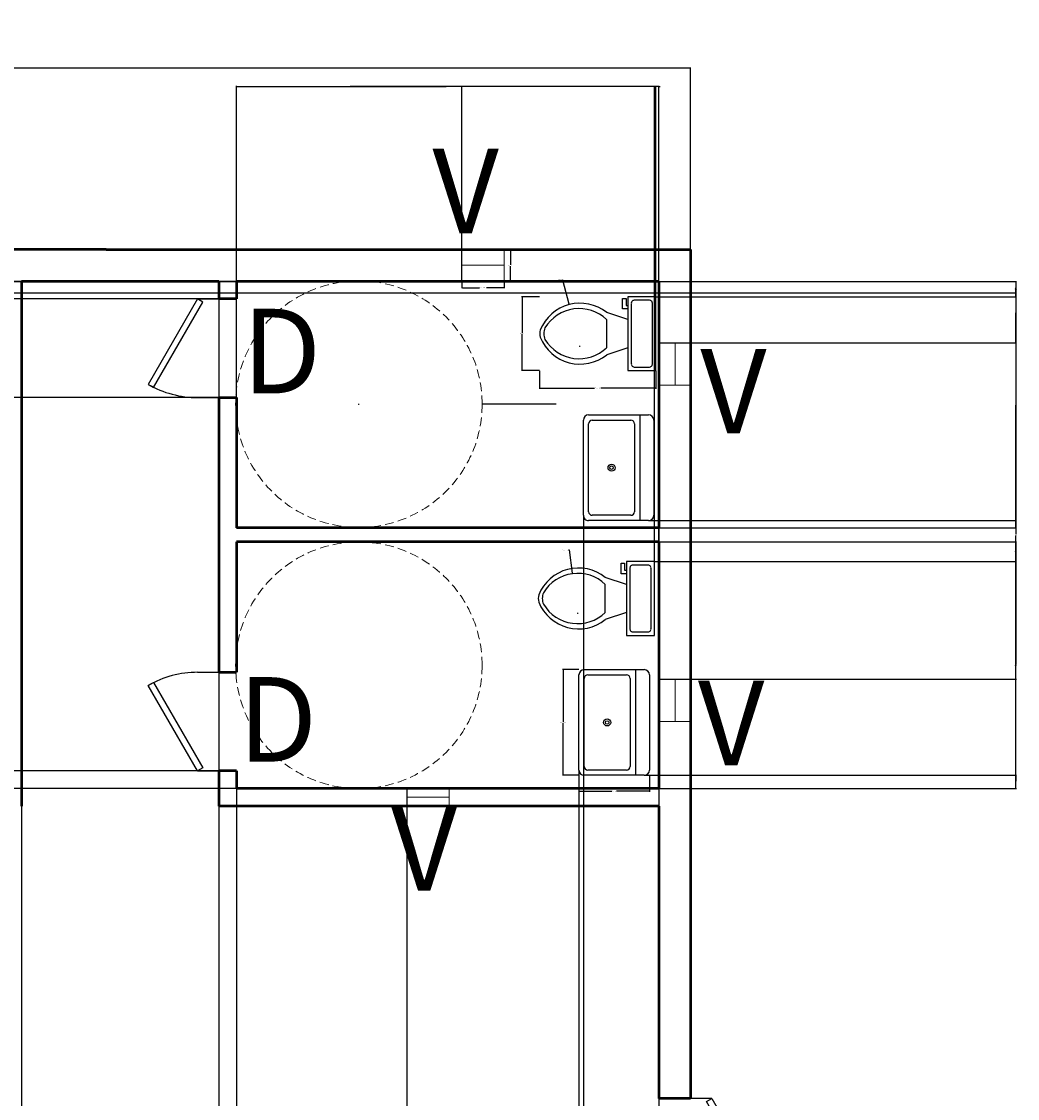
# Model space of a CAD drawing. Units: inches. Extents: x -84 to 931, y 65 to 668.
# Tile 5 of 5: x 649 to 931, y 363 to 668. Entities that reach past the tile are written whole.
import ezdxf

# ---------------------------------------------------------------- set-up
doc = ezdxf.new("R2010")
doc.units = ezdxf.units.IN
doc.header["$MEASUREMENT"] = 0
doc.linetypes.add('HIDDEN', pattern=[0.375, 0.25, -0.125])
for name, color, linetype, lineweight in [('A-ANNO-DIMS', 2, 'Continuous', 18), ('A-ANNO-TEXT', 7, 'Continuous', 18), ('A-DOOR', 4, 'Continuous', 25), ('A-FLOR-CLRN', 8, 'HIDDEN', 13), ('A-FLOR-FIXT', 9, 'Continuous', 25), ('A-GLAZ-VENT', 3, 'Continuous', 18), ('A-WALL', 7, 'Continuous', 50)]:
    doc.layers.add(name, color=color, linetype=linetype, lineweight=lineweight)
doc.styles.get("Standard").update_dxf_attribs({"font": 'arial.ttf'})
doc.dimstyles.get("Standard").update_dxf_attribs({"dimtxt": 0.18, "dimasz": 0.18, "dimexe": 0.18, "dimexo": 0.0625, "dimgap": 0.09, "dimtad": 0, "dimtih": 1, "dimtoh": 1, "dimdec": 0, "dimzin": 0, "dimdsep": 46, "dimlunit": 3, "dimtxsty": 'Standard', "dimcen": 0.09, "dimadec": 0, "dimazin": 0, "dimtfac": 1, "dimtdec": 0, "dimtofl": 0, "dimtmove": 0, "dimatfit": 3, "dimfxl": 1, "dimtolj": 1, "dimtzin": 0, "dimarcsym": 0})

# ---------------------------------------------------------------- blocks, each defined once
blk = doc.blocks.new('*U5')
for p, q in [((0, 0), (0, -6)), ((-28, 0), (-28, -6))]:
    blk.add_line(p, q)
blk.add_lwpolyline([(0, 0), (-24.25, 14), (-25.12, 12.48), (-0.87, -1.52)], close=True)
blk.add_arc((0, 0), 28, 150, 180)
blk = doc.blocks.new('*U6')
for p, q in [((0, 0), (0, -6)), ((28, 0), (28, -6))]:
    blk.add_line(p, q)
blk.add_lwpolyline([(0, 0), (24.25, 14), (25.12, 12.48), (0.87, -1.52)], close=True)
blk.add_arc((0, 0), 28, 0, 30)
blk = doc.blocks.new('*U13')
for p, q in [((-40, 0), (-40, 6)), ((0, 0), (0, 6))]:
    blk.add_line(p, q)
blk.add_lwpolyline([(0, 0), (-34.64, -20), (-35.52, -18.48), (-0.87, 1.52)], close=True)
blk.add_arc((0, 0), 40, 180, 210)
blk = doc.blocks.new('Sink-single - 30 in top')
blk.add_line((-15, -3.999996), (15, -3.999996))
for points in [[(-13.5, 0), (13.5, 0)], [(-15, -18.499996), (-15, -1.5)], [(15, -1.5), (15, -18.499996)], [(-12.5, -5.499996), (12.5, -5.499996)], [(-13.5, -17.499996), (-13.5, -6.499996)], [(13.5, -6.499996), (13.5, -17.499996)], [(13.5, -19.999996), (-13.5, -19.999996)], [(12.5, -18.499996), (-12.5, -18.499996)]]:
    blk.add_lwpolyline(points)
for radius in [1, 0.5]:
    blk.add_circle((0, -11.999996), radius)
for centre, radius, start, end in [((-13.5, -1.5), 1.5, 90, 180), ((13.5, -1.5), 1.5, 0, 90), ((-12.5, -6.499996), 1, 90, 180), ((12.5, -6.499996), 1, 0, 90), ((-12.5, -17.499996), 1, 180, 270), ((12.5, -17.499996), 1, 270, 0), ((-13.5, -18.499996), 1.5, 180, 270), ((13.5, -18.499996), 1.5, 270, 0)]:
    blk.add_arc(centre, radius, start, end)
blk = doc.blocks.new('Toilet - top')
for p, q in [((9.5, -6), (9.5, -2)), ((-10, -8.5), (-8, -8.5)), ((-10, -9.5), (-10, -8.5)), ((-8, -8.5), (-8, -8)), ((-7, -8), (-7, -9.5)), ((-4, -8), (-6, -14)), ((4, -8), (6, -14)), ((-7, -9.5), (-10, -9.5)), ((4, -14), (-4, -14))]:
    blk.add_line(p, q)
blk.add_lwpolyline([(10.5, -8), (10.5, 0), (-10.5, 0), (-10.5, -8)], close=True)
for points in [[(-9.5, -2), (-9.5, -6)], [(8.5, -1), (-8.5, -1)], [(-8.5, -7), (8.5, -7)]]:
    blk.add_lwpolyline(points)
for centre, radius, start, end in [((-8.62, -1.88), 0.884, 81.8699, 188.1301), ((8.62, -1.88), 0.884, 351.8699, 98.1301), ((-8.62, -6.12), 0.884, 171.8699, 278.1301), ((8.62, -6.12), 0.884, 261.8699, 8.1301), ((3.52, -21.58), 12.17, 141.4691, 247.9714), ((4.2, -21.82), 11.33, 136.3677, 238.9468), ((-3.52, -21.58), 12.17, 292.0284, 38.5307), ((-4.2, -21.82), 11.33, 301.053, 43.6321), ((0, -27.88), 4, 245.7318, 294.2682), ((0, -29), 4, 254.8605, 285.1395)]:
    blk.add_arc(centre, radius, start, end)
blk = doc.blocks.new('*D17')
at = {"layer": 'A-ANNO-DIMS', "color": 0, "lineweight": -2, "transparency": 16777216}
for p, q in [((0.53, 603.58), (0.53, 655.22)), ((0.71, 655.04), (368.83, 655.04)), ((838.35, 655.04), (470.23, 655.04)), ((838.53, 603.58), (838.53, 655.22))]:
    blk.add_line(p, q, dxfattribs=at)
at = {"layer": 'A-ANNO-DIMS', "color": 0, "transparency": 16777216}
for points in [[(0.71, 655.07), (0.71, 655.01), (0.53, 655.04)], [(838.35, 655.07), (838.35, 655.01), (838.53, 655.04)]]:
    blk.add_solid(points, dxfattribs=at)
at = {"layer": 'Defpoints', "color": 0, "transparency": 16777216}
for p in [(838.53, 655.04), (0.53, 603.52), (838.53, 603.52)]:
    blk.add_point(p, dxfattribs=at)
at = {"layer": 'A-ANNO-DIMS', "color": 0, "transparency": 16777216, "insert": (419.53, 655.04), "char_height": 0.18, "attachment_point": 5}
blk.add_mtext('\\A1;{\\H133.33333x;69\'-10"}', dxfattribs=at)
blk = doc.blocks.new('VENT-12IN-EXT')
blk.add_line((0, 4.61), (12, 4.61))
blk.add_lwpolyline([(0, 9), (12, 9), (12, 0), (0, 0)], close=True)
blk = doc.blocks.new('*D23')
at = {"layer": 'A-ANNO-DIMS', "color": 0, "lineweight": -2, "transparency": 16777216}
for p, q in [((795.65, 569.11), (795.65, 564.04)), ((828.69, 569.11), (828.69, 564.04)), ((795.83, 564.22), (811.28, 564.22)), ((828.51, 564.22), (813.06, 564.22))]:
    blk.add_line(p, q, dxfattribs=at)
at = {"layer": 'A-ANNO-DIMS', "color": 0, "transparency": 16777216}
for points in [[(795.83, 564.25), (795.83, 564.19), (795.65, 564.22)], [(828.51, 564.25), (828.51, 564.19), (828.69, 564.22)]]:
    blk.add_solid(points, dxfattribs=at)
at = {"layer": 'Defpoints', "color": 0, "transparency": 16777216}
for p in [(795.65, 569.17), (828.69, 569.17), (828.69, 564.22)]:
    blk.add_point(p, dxfattribs=at)
at = {"layer": 'A-ANNO-DIMS', "color": 0, "transparency": 16777216, "insert": (812.17, 564.22), "char_height": 0.18, "attachment_point": 5}
blk.add_mtext('\\A1;WC 2\'-9" TYP.', dxfattribs=at)
blk = doc.blocks.new('*D24')
at = {"layer": 'A-ANNO-DIMS', "color": 0, "lineweight": -2, "transparency": 16777216}
for p, q in [((795.58, 590.17), (790.51, 590.17)), ((790.69, 589.99), (790.69, 579.85)), ((790.69, 569.35), (790.69, 579.49)), ((795.58, 569.17), (790.51, 569.17))]:
    blk.add_line(p, q, dxfattribs=at)
at = {"layer": 'A-ANNO-DIMS', "color": 0, "transparency": 16777216}
for points in [[(790.66, 589.99), (790.72, 589.99), (790.69, 590.17)], [(790.66, 569.35), (790.72, 569.35), (790.69, 569.17)]]:
    blk.add_solid(points, dxfattribs=at)
at = {"layer": 'Defpoints', "color": 0, "transparency": 16777216}
for p in [(795.65, 590.17), (790.69, 569.17), (795.65, 569.17)]:
    blk.add_point(p, dxfattribs=at)
at = {"layer": 'A-ANNO-DIMS', "color": 0, "transparency": 16777216, "insert": (790.69, 579.67), "char_height": 0.18, "attachment_point": 5}
blk.add_mtext('\\A1;1\'-9" TYP.', dxfattribs=at)
blk = doc.blocks.new('*D25')
at = {"layer": 'A-ANNO-DIMS', "color": 0, "lineweight": -2, "transparency": 16777216}
for p, q in [((773.54, 594.45), (773.54, 592.54)), ((785.54, 594.45), (785.54, 592.54)), ((773.72, 592.72), (778.53, 592.72)), ((785.36, 592.72), (780.55, 592.72))]:
    blk.add_line(p, q, dxfattribs=at)
at = {"layer": 'A-ANNO-DIMS', "color": 0, "transparency": 16777216}
for points in [[(773.72, 592.75), (773.72, 592.69), (773.54, 592.72)], [(785.36, 592.75), (785.36, 592.69), (785.54, 592.72)]]:
    blk.add_solid(points, dxfattribs=at)
at = {"layer": 'Defpoints', "color": 0, "transparency": 16777216}
for p in [(773.54, 594.52), (785.54, 594.52), (785.54, 592.72)]:
    blk.add_point(p, dxfattribs=at)
at = {"layer": 'A-ANNO-DIMS', "color": 0, "transparency": 16777216, "insert": (779.54, 592.72), "char_height": 0.18, "attachment_point": 5}
blk.add_mtext('\\A1;VENT 1\'-0" TYP.', dxfattribs=at)
blk = doc.blocks.new('*D26')
at = {"layer": 'A-ANNO-DIMS', "color": 0, "lineweight": -2, "transparency": 16777216}
for p, q in [((785.6, 603.52), (787.52, 603.52)), ((787.34, 603.34), (787.34, 599.2)), ((787.34, 594.7), (787.34, 598.83)), ((785.6, 594.52), (787.52, 594.52))]:
    blk.add_line(p, q, dxfattribs=at)
at = {"layer": 'A-ANNO-DIMS', "color": 0, "transparency": 16777216}
for points in [[(787.31, 603.34), (787.37, 603.34), (787.34, 603.52)], [(787.31, 594.7), (787.37, 594.7), (787.34, 594.52)]]:
    blk.add_solid(points, dxfattribs=at)
at = {"layer": 'Defpoints', "color": 0, "transparency": 16777216}
for p in [(785.54, 603.52), (787.34, 603.52), (785.54, 594.52)]:
    blk.add_point(p, dxfattribs=at)
at = {"layer": 'A-ANNO-DIMS', "color": 0, "transparency": 16777216, "insert": (787.34, 599.02), "char_height": 0.18, "attachment_point": 5}
blk.add_mtext('\\A1;0\'-9" TYP.', dxfattribs=at)
blk = doc.blocks.new('*D27')
at = {"layer": 'A-ANNO-DIMS', "color": 0, "lineweight": -2, "transparency": 16777216}
for p, q in [((806.77, 484.27), (802.15, 484.27)), ((802.33, 484.09), (802.33, 469.45)), ((802.33, 454.45), (802.33, 469.08)), ((806.77, 454.27), (802.15, 454.27))]:
    blk.add_line(p, q, dxfattribs=at)
at = {"layer": 'A-ANNO-DIMS', "color": 0, "transparency": 16777216}
for points in [[(802.3, 484.09), (802.36, 484.09), (802.33, 484.27)], [(802.3, 454.45), (802.36, 454.45), (802.33, 454.27)]]:
    blk.add_solid(points, dxfattribs=at)
at = {"layer": 'Defpoints', "color": 0, "transparency": 16777216}
for p in [(806.83, 484.27), (802.33, 454.27), (806.83, 454.27)]:
    blk.add_point(p, dxfattribs=at)
at = {"layer": 'A-ANNO-DIMS', "color": 0, "transparency": 16777216, "insert": (802.33, 469.27), "char_height": 0.18, "attachment_point": 5}
blk.add_mtext('\\A1;BASIN 2\'-6" TYP.', dxfattribs=at)
blk = doc.blocks.new('*D28')
at = {"layer": 'A-ANNO-DIMS', "color": 0, "lineweight": -2, "transparency": 16777216}
for p, q in [((806.83, 454.2), (806.83, 449.59)), ((826.83, 454.2), (826.83, 449.59)), ((807.01, 449.77), (816.2, 449.77)), ((826.65, 449.77), (817.46, 449.77))]:
    blk.add_line(p, q, dxfattribs=at)
at = {"layer": 'A-ANNO-DIMS', "color": 0, "transparency": 16777216}
for points in [[(807.01, 449.8), (807.01, 449.74), (806.83, 449.77)], [(826.65, 449.8), (826.65, 449.74), (826.83, 449.77)]]:
    blk.add_solid(points, dxfattribs=at)
at = {"layer": 'Defpoints', "color": 0, "transparency": 16777216}
for p in [(806.83, 454.27), (826.83, 454.27), (826.83, 449.77)]:
    blk.add_point(p, dxfattribs=at)
at = {"layer": 'A-ANNO-DIMS', "color": 0, "transparency": 16777216, "insert": (816.83, 449.77), "char_height": 0.18, "attachment_point": 5}
blk.add_mtext('\\A1;1\'-8" TYP.', dxfattribs=at)
blk = doc.blocks.new('*D39')
at = {"layer": 'A-ANNO-DIMS', "color": 0, "lineweight": -2, "transparency": 16777216}
for p, q in [((648.53, 594.45), (648.53, 64.99)), ((704.53, 594.45), (704.53, 64.99)), ((648.71, 65.17), (676.2, 65.17)), ((704.35, 65.17), (676.86, 65.17))]:
    blk.add_line(p, q, dxfattribs=at)
at = {"layer": 'A-ANNO-DIMS', "color": 0, "transparency": 16777216}
for points in [[(648.71, 65.2), (648.71, 65.14), (648.53, 65.17)], [(704.35, 65.2), (704.35, 65.14), (704.53, 65.17)]]:
    blk.add_solid(points, dxfattribs=at)
at = {"layer": 'Defpoints', "color": 0, "transparency": 16777216}
for p in [(648.53, 594.52), (704.53, 594.52), (704.53, 65.17)]:
    blk.add_point(p, dxfattribs=at)
at = {"layer": 'A-ANNO-DIMS', "color": 0, "transparency": 16777216, "insert": (676.53, 65.17), "char_height": 0.18, "attachment_point": 5}
blk.add_mtext('\\A1;4\'-8"', dxfattribs=at)
blk = doc.blocks.new('*D40')
at = {"layer": 'A-ANNO-DIMS', "color": 0, "lineweight": -2, "transparency": 16777216}
for p, q in [((709.53, 524.58), (709.53, 650.05)), ((709.71, 649.87), (769.14, 649.87)), ((829.35, 649.87), (769.92, 649.87)), ((829.53, 524.58), (829.53, 650.05))]:
    blk.add_line(p, q, dxfattribs=at)
at = {"layer": 'A-ANNO-DIMS', "color": 0, "transparency": 16777216}
for points in [[(709.71, 649.9), (709.71, 649.84), (709.53, 649.87)], [(829.35, 649.9), (829.35, 649.84), (829.53, 649.87)]]:
    blk.add_solid(points, dxfattribs=at)
at = {"layer": 'Defpoints', "color": 0, "transparency": 16777216}
for p in [(829.53, 649.87), (709.53, 524.52), (829.53, 524.52)]:
    blk.add_point(p, dxfattribs=at)
at = {"layer": 'A-ANNO-DIMS', "color": 0, "transparency": 16777216, "insert": (769.53, 649.87), "char_height": 0.18, "attachment_point": 5}
blk.add_mtext('\\A1;10\'-0"', dxfattribs=at)
blk = doc.blocks.new('*D49')
at = {"layer": 'A-ANNO-DIMS', "color": 0, "lineweight": -2, "transparency": 16777216}
for p, q in [((829.59, 594.52), (931.06, 594.52)), ((930.88, 594.34), (930.88, 559.7)), ((930.88, 524.7), (930.88, 559.33)), ((829.59, 524.52), (931.06, 524.52))]:
    blk.add_line(p, q, dxfattribs=at)
at = {"layer": 'A-ANNO-DIMS', "color": 0, "transparency": 16777216}
for points in [[(930.85, 594.34), (930.91, 594.34), (930.88, 594.52)], [(930.85, 524.7), (930.91, 524.7), (930.88, 524.52)]]:
    blk.add_solid(points, dxfattribs=at)
at = {"layer": 'Defpoints', "color": 0, "transparency": 16777216}
for p in [(829.53, 594.52), (829.53, 524.52), (930.88, 524.52)]:
    blk.add_point(p, dxfattribs=at)
at = {"layer": 'A-ANNO-DIMS', "color": 0, "transparency": 16777216, "insert": (930.88, 559.52), "char_height": 0.18, "attachment_point": 5}
blk.add_mtext('\\A1;5\'-10"', dxfattribs=at)
blk = doc.blocks.new('*D50')
at = {"layer": 'A-ANNO-DIMS', "color": 0, "lineweight": -2, "transparency": 16777216}
for p, q in [((829.59, 520.52), (931.06, 520.52)), ((930.88, 520.34), (930.88, 485.7)), ((930.88, 450.7), (930.88, 485.33)), ((829.59, 450.52), (931.06, 450.52))]:
    blk.add_line(p, q, dxfattribs=at)
at = {"layer": 'A-ANNO-DIMS', "color": 0, "transparency": 16777216}
for points in [[(930.85, 520.34), (930.91, 520.34), (930.88, 520.52)], [(930.85, 450.7), (930.91, 450.7), (930.88, 450.52)]]:
    blk.add_solid(points, dxfattribs=at)
at = {"layer": 'Defpoints', "color": 0, "transparency": 16777216}
for p in [(829.53, 520.52), (829.53, 450.52), (930.88, 450.52)]:
    blk.add_point(p, dxfattribs=at)
at = {"layer": 'A-ANNO-DIMS', "color": 0, "transparency": 16777216, "insert": (930.88, 485.52), "char_height": 0.18, "attachment_point": 5}
blk.add_mtext('\\A1;5\'-10"', dxfattribs=at)
blk = doc.blocks.new('*D55')
at = {"layer": 'A-ANNO-DIMS', "color": 0, "lineweight": -2, "transparency": 16777216}
for p, q in [((704.47, 589.52), (-84, 589.52)), ((-83.82, 589.34), (-83.82, 575.7)), ((-83.82, 561.7), (-83.82, 575.34)), ((704.47, 561.52), (-84, 561.52))]:
    blk.add_line(p, q, dxfattribs=at)
at = {"layer": 'A-ANNO-DIMS', "color": 0, "transparency": 16777216}
for points in [[(-83.85, 589.34), (-83.79, 589.34), (-83.82, 589.52)], [(-83.85, 561.7), (-83.79, 561.7), (-83.82, 561.52)]]:
    blk.add_solid(points, dxfattribs=at)
at = {"layer": 'Defpoints', "color": 0, "transparency": 16777216}
for p in [(-83.82, 589.52), (704.53, 589.52), (704.53, 561.52)]:
    blk.add_point(p, dxfattribs=at)
at = {"layer": 'A-ANNO-DIMS', "color": 0, "transparency": 16777216, "insert": (-83.82, 575.52), "char_height": 0.18, "attachment_point": 5}
blk.add_mtext('\\A1;2\'-4"', dxfattribs=at)
blk = doc.blocks.new('*D62')
at = {"layer": 'A-ANNO-DIMS', "color": 0, "lineweight": -2, "transparency": 16777216}
for p, q in [((643.59, 594.52), (931.06, 594.52)), ((930.88, 594.34), (930.88, 522.7)), ((930.88, 450.7), (930.88, 522.33)), ((829.59, 450.52), (931.06, 450.52))]:
    blk.add_line(p, q, dxfattribs=at)
at = {"layer": 'A-ANNO-DIMS', "color": 0, "transparency": 16777216}
for points in [[(930.85, 594.34), (930.91, 594.34), (930.88, 594.52)], [(930.85, 450.7), (930.91, 450.7), (930.88, 450.52)]]:
    blk.add_solid(points, dxfattribs=at)
at = {"layer": 'Defpoints', "color": 0, "transparency": 16777216}
for p in [(643.53, 594.52), (829.53, 450.52), (930.88, 450.52)]:
    blk.add_point(p, dxfattribs=at)
at = {"layer": 'A-ANNO-DIMS', "color": 0, "transparency": 16777216, "insert": (930.88, 522.52), "char_height": 0.18, "attachment_point": 5}
blk.add_mtext('\\A1;12\'-0"', dxfattribs=at)
blk = doc.blocks.new('*D65')
at = {"layer": 'A-ANNO-DIMS', "color": 0, "lineweight": -2, "transparency": 16777216}
for p, q in [((829.59, 594.52), (931.06, 594.52)), ((930.88, 594.34), (930.88, 585.98)), ((930.88, 577.27), (930.88, 585.62)), ((829.59, 577.09), (931.06, 577.09))]:
    blk.add_line(p, q, dxfattribs=at)
at = {"layer": 'A-ANNO-DIMS', "color": 0, "transparency": 16777216}
for points in [[(930.85, 594.34), (930.91, 594.34), (930.88, 594.52)], [(930.85, 577.27), (930.91, 577.27), (930.88, 577.09)]]:
    blk.add_solid(points, dxfattribs=at)
at = {"layer": 'Defpoints', "color": 0, "transparency": 16777216}
for p in [(829.53, 594.52), (930.88, 594.52), (829.53, 577.09)]:
    blk.add_point(p, dxfattribs=at)
at = {"layer": 'A-ANNO-DIMS', "color": 0, "transparency": 16777216, "insert": (930.88, 585.8), "char_height": 0.18, "attachment_point": 5}
blk.add_mtext('\\A1;1\'-5 1/2"', dxfattribs=at)
blk = doc.blocks.new('*D66')
at = {"layer": 'A-ANNO-DIMS', "color": 0, "lineweight": -2, "transparency": 16777216}
for p, q in [((829.59, 520.52), (931.06, 520.52)), ((930.88, 520.34), (930.88, 501.22)), ((930.88, 481.75), (930.88, 500.86)), ((829.59, 481.57), (931.06, 481.57))]:
    blk.add_line(p, q, dxfattribs=at)
at = {"layer": 'A-ANNO-DIMS', "color": 0, "transparency": 16777216}
for points in [[(930.85, 520.34), (930.91, 520.34), (930.88, 520.52)], [(930.85, 481.75), (930.91, 481.75), (930.88, 481.57)]]:
    blk.add_solid(points, dxfattribs=at)
at = {"layer": 'Defpoints', "color": 0, "transparency": 16777216}
for p in [(829.53, 520.52), (930.88, 520.52), (829.53, 481.57)]:
    blk.add_point(p, dxfattribs=at)
at = {"layer": 'A-ANNO-DIMS', "color": 0, "transparency": 16777216, "insert": (930.88, 501.04), "char_height": 0.18, "attachment_point": 5}
blk.add_mtext('\\A1;3\'-3"', dxfattribs=at)
blk = doc.blocks.new('*D67')
at = {"layer": 'A-ANNO-DIMS', "color": 0, "lineweight": -2, "transparency": 16777216}
for p, q in [((709.53, 594.58), (709.53, 650.05)), ((709.71, 649.87), (741.21, 649.87)), ((773.36, 649.87), (741.86, 649.87)), ((773.54, 594.58), (773.54, 650.05))]:
    blk.add_line(p, q, dxfattribs=at)
at = {"layer": 'A-ANNO-DIMS', "color": 0, "transparency": 16777216}
for points in [[(709.71, 649.9), (709.71, 649.84), (709.53, 649.87)], [(773.36, 649.9), (773.36, 649.84), (773.54, 649.87)]]:
    blk.add_solid(points, dxfattribs=at)
at = {"layer": 'Defpoints', "color": 0, "transparency": 16777216}
for p in [(773.54, 649.87), (709.53, 594.52), (773.54, 594.52)]:
    blk.add_point(p, dxfattribs=at)
at = {"layer": 'A-ANNO-DIMS', "color": 0, "transparency": 16777216, "insert": (741.54, 649.87), "char_height": 0.18, "attachment_point": 5}
blk.add_mtext('\\A1;5\'-4"', dxfattribs=at)
blk = doc.blocks.new('*D68')
at = {"layer": 'A-ANNO-DIMS', "color": 0, "lineweight": -2, "transparency": 16777216}
for p, q in [((709.53, 450.45), (709.53, 64.99)), ((757.92, 450.45), (757.92, 64.99)), ((709.71, 65.17), (733.18, 65.17)), ((757.74, 65.17), (734.27, 65.17))]:
    blk.add_line(p, q, dxfattribs=at)
at = {"layer": 'A-ANNO-DIMS', "color": 0, "transparency": 16777216}
for points in [[(709.71, 65.2), (709.71, 65.14), (709.53, 65.17)], [(757.74, 65.2), (757.74, 65.14), (757.92, 65.17)]]:
    blk.add_solid(points, dxfattribs=at)
at = {"layer": 'Defpoints', "color": 0, "transparency": 16777216}
for p in [(709.53, 450.52), (757.92, 450.52), (757.92, 65.17)]:
    blk.add_point(p, dxfattribs=at)
at = {"layer": 'A-ANNO-DIMS', "color": 0, "transparency": 16777216, "insert": (733.73, 65.17), "char_height": 0.18, "attachment_point": 5}
blk.add_mtext('\\A1;4\'-0 1/2"', dxfattribs=at)
blk = doc.blocks.new('*D76')
at = {"layer": 'A-ANNO-DIMS', "color": 0, "lineweight": -2, "transparency": 16777216}
for p, q in [((297.59, 594.52), (931.06, 594.52)), ((930.88, 594.34), (930.88, 593.09)), ((263.98, 591.29), (931.06, 591.29)), ((930.88, 591.47), (930.88, 592.72))]:
    blk.add_line(p, q, dxfattribs=at)
at = {"layer": 'A-ANNO-DIMS', "color": 0, "transparency": 16777216}
for points in [[(930.85, 594.34), (930.91, 594.34), (930.88, 594.52)], [(930.85, 591.47), (930.91, 591.47), (930.88, 591.29)]]:
    blk.add_solid(points, dxfattribs=at)
at = {"layer": 'Defpoints', "color": 0, "transparency": 16777216}
for p in [(297.53, 594.52), (930.88, 594.52), (263.92, 591.29)]:
    blk.add_point(p, dxfattribs=at)
at = {"layer": 'A-ANNO-DIMS', "color": 0, "transparency": 16777216, "insert": (930.88, 592.9), "char_height": 0.18, "attachment_point": 5}
blk.add_mtext('\\A1;0\'-3"', dxfattribs=at)
blk = doc.blocks.new('*D79')
at = {"layer": 'A-ANNO-DIMS', "color": 0, "lineweight": -2, "transparency": 16777216}
for p, q in [((829.59, 594.52), (931.06, 594.52)), ((930.88, 594.34), (930.88, 592.53)), ((828.76, 590.17), (931.06, 590.17)), ((930.88, 590.35), (930.88, 592.16))]:
    blk.add_line(p, q, dxfattribs=at)
at = {"layer": 'A-ANNO-DIMS', "color": 0, "transparency": 16777216}
for points in [[(930.85, 594.34), (930.91, 594.34), (930.88, 594.52)], [(930.85, 590.35), (930.91, 590.35), (930.88, 590.17)]]:
    blk.add_solid(points, dxfattribs=at)
at = {"layer": 'Defpoints', "color": 0, "transparency": 16777216}
for p in [(829.53, 594.52), (930.88, 594.52), (828.69, 590.17)]:
    blk.add_point(p, dxfattribs=at)
at = {"layer": 'A-ANNO-DIMS', "color": 0, "transparency": 16777216, "insert": (930.88, 592.34), "char_height": 0.18, "attachment_point": 5}
blk.add_mtext('\\A1;0\'-4 1/2"', dxfattribs=at)
blk = doc.blocks.new('*D80')
at = {"layer": 'A-ANNO-DIMS', "color": 0, "lineweight": -2, "transparency": 16777216}
for p, q in [((829.59, 520.52), (931.06, 520.52)), ((930.88, 520.34), (930.88, 517.93)), ((930.88, 515.16), (930.88, 517.57)), ((828.34, 514.98), (931.06, 514.98))]:
    blk.add_line(p, q, dxfattribs=at)
at = {"layer": 'A-ANNO-DIMS', "color": 0, "transparency": 16777216}
for points in [[(930.85, 520.34), (930.91, 520.34), (930.88, 520.52)], [(930.85, 515.16), (930.91, 515.16), (930.88, 514.98)]]:
    blk.add_solid(points, dxfattribs=at)
at = {"layer": 'Defpoints', "color": 0, "transparency": 16777216}
for p in [(829.53, 520.52), (930.88, 520.52), (828.28, 514.98)]:
    blk.add_point(p, dxfattribs=at)
at = {"layer": 'A-ANNO-DIMS', "color": 0, "transparency": 16777216, "insert": (930.88, 517.75), "char_height": 0.18, "attachment_point": 5}
blk.add_mtext('\\A1;0\'-5 1/2"', dxfattribs=at)
blk = doc.blocks.new('*D81')
at = {"layer": 'A-ANNO-DIMS', "color": 0, "lineweight": -2, "transparency": 16777216}
for p, q in [((826.64, 526.6), (931.06, 526.6)), ((930.88, 526.42), (930.88, 525.74)), ((829.59, 524.52), (931.06, 524.52)), ((930.88, 524.7), (930.88, 525.38))]:
    blk.add_line(p, q, dxfattribs=at)
at = {"layer": 'A-ANNO-DIMS', "color": 0, "transparency": 16777216}
for points in [[(930.85, 526.42), (930.91, 526.42), (930.88, 526.6)], [(930.85, 524.7), (930.91, 524.7), (930.88, 524.52)]]:
    blk.add_solid(points, dxfattribs=at)
at = {"layer": 'Defpoints', "color": 0, "transparency": 16777216}
for p in [(826.57, 526.6), (829.53, 524.52), (930.88, 524.52)]:
    blk.add_point(p, dxfattribs=at)
at = {"layer": 'A-ANNO-DIMS', "color": 0, "transparency": 16777216, "insert": (930.88, 525.56), "char_height": 0.18, "attachment_point": 5}
blk.add_mtext('\\A1;0\'-2"', dxfattribs=at)
blk = doc.blocks.new('*D82')
at = {"layer": 'A-ANNO-DIMS', "color": 0, "lineweight": -2, "transparency": 16777216}
for p, q in [((825.4, 454.27), (931.06, 454.27)), ((930.88, 454.09), (930.88, 452.57)), ((829.59, 450.52), (931.06, 450.52)), ((930.88, 450.7), (930.88, 452.21))]:
    blk.add_line(p, q, dxfattribs=at)
at = {"layer": 'A-ANNO-DIMS', "color": 0, "transparency": 16777216}
for points in [[(930.85, 454.09), (930.91, 454.09), (930.88, 454.27)], [(930.85, 450.7), (930.91, 450.7), (930.88, 450.52)]]:
    blk.add_solid(points, dxfattribs=at)
at = {"layer": 'Defpoints', "color": 0, "transparency": 16777216}
for p in [(825.33, 454.27), (829.53, 450.52), (930.88, 450.52)]:
    blk.add_point(p, dxfattribs=at)
at = {"layer": 'A-ANNO-DIMS', "color": 0, "transparency": 16777216, "insert": (930.88, 452.39), "char_height": 0.18, "attachment_point": 5}
blk.add_mtext('\\A1;0\'-4"', dxfattribs=at)
blk = doc.blocks.new('*D83')
at = {"layer": 'A-ANNO-DIMS', "color": 0, "lineweight": -2, "transparency": 16777216}
for p, q in [((709.47, 594.52), (-84, 594.52)), ((-83.82, 594.34), (-83.82, 592.2)), ((-83.82, 589.7), (-83.82, 591.83)), ((709.47, 589.52), (-84, 589.52))]:
    blk.add_line(p, q, dxfattribs=at)
at = {"layer": 'A-ANNO-DIMS', "color": 0, "transparency": 16777216}
for points in [[(-83.85, 594.34), (-83.79, 594.34), (-83.82, 594.52)], [(-83.85, 589.7), (-83.79, 589.7), (-83.82, 589.52)]]:
    blk.add_solid(points, dxfattribs=at)
at = {"layer": 'Defpoints', "color": 0, "transparency": 16777216}
for p in [(-83.82, 594.52), (709.53, 594.52), (709.53, 589.52)]:
    blk.add_point(p, dxfattribs=at)
at = {"layer": 'A-ANNO-DIMS', "color": 0, "transparency": 16777216, "insert": (-83.82, 592.02), "char_height": 0.18, "attachment_point": 5}
blk.add_mtext('\\A1;0\'-5"', dxfattribs=at)
blk = doc.blocks.new('*D84')
at = {"layer": 'A-ANNO-DIMS', "color": 0, "lineweight": -2, "transparency": 16777216}
for p, q in [((709.47, 455.52), (-84, 455.52)), ((-83.82, 455.34), (-83.82, 453.2)), ((-83.82, 450.7), (-83.82, 452.83)), ((709.47, 450.52), (-84, 450.52))]:
    blk.add_line(p, q, dxfattribs=at)
at = {"layer": 'A-ANNO-DIMS', "color": 0, "transparency": 16777216}
for points in [[(-83.85, 455.34), (-83.79, 455.34), (-83.82, 455.52)], [(-83.85, 450.7), (-83.79, 450.7), (-83.82, 450.52)]]:
    blk.add_solid(points, dxfattribs=at)
at = {"layer": 'Defpoints', "color": 0, "transparency": 16777216}
for p in [(709.53, 455.52), (-83.82, 450.52), (709.53, 450.52)]:
    blk.add_point(p, dxfattribs=at)
at = {"layer": 'A-ANNO-DIMS', "color": 0, "transparency": 16777216, "insert": (-83.82, 453.02), "char_height": 0.18, "attachment_point": 5}
blk.add_mtext('\\A1;0\'-5"', dxfattribs=at)
blk = doc.blocks.new('*D89')
at = {"layer": 'A-ANNO-DIMS', "color": 0, "lineweight": -2, "transparency": 16777216}
for p, q in [((808.07, 528.04), (808.07, 64.99)), ((829.53, 524.45), (829.53, 64.99)), ((808.25, 65.17), (818.27, 65.17)), ((829.35, 65.17), (819.33, 65.17))]:
    blk.add_line(p, q, dxfattribs=at)
at = {"layer": 'A-ANNO-DIMS', "color": 0, "transparency": 16777216}
for points in [[(808.25, 65.2), (808.25, 65.14), (808.07, 65.17)], [(829.35, 65.2), (829.35, 65.14), (829.53, 65.17)]]:
    blk.add_solid(points, dxfattribs=at)
at = {"layer": 'Defpoints', "color": 0, "transparency": 16777216}
for p in [(808.07, 528.1), (829.53, 524.52), (829.53, 65.17)]:
    blk.add_point(p, dxfattribs=at)
at = {"layer": 'A-ANNO-DIMS', "color": 0, "transparency": 16777216, "insert": (818.8, 65.17), "char_height": 0.18, "attachment_point": 5}
blk.add_mtext('\\A1;1\'-9 1/2"', dxfattribs=at)
blk = doc.blocks.new('*D90')
at = {"layer": 'A-ANNO-DIMS', "color": 0, "lineweight": -2, "transparency": 16777216}
for p, q in [((806.83, 455.7), (806.83, 64.99)), ((829.53, 450.45), (829.53, 64.99)), ((807.01, 65.17), (817.58, 65.17)), ((829.35, 65.17), (818.78, 65.17))]:
    blk.add_line(p, q, dxfattribs=at)
at = {"layer": 'A-ANNO-DIMS', "color": 0, "transparency": 16777216}
for points in [[(807.01, 65.2), (807.01, 65.14), (806.83, 65.17)], [(829.35, 65.2), (829.35, 65.14), (829.53, 65.17)]]:
    blk.add_solid(points, dxfattribs=at)
at = {"layer": 'Defpoints', "color": 0, "transparency": 16777216}
for p in [(806.83, 455.77), (829.53, 450.52), (829.53, 65.17)]:
    blk.add_point(p, dxfattribs=at)
at = {"layer": 'A-ANNO-DIMS', "color": 0, "transparency": 16777216, "insert": (818.18, 65.17), "char_height": 0.18, "attachment_point": 5}
blk.add_mtext('\\A1;1\'-10 1/2"', dxfattribs=at)
blk = doc.blocks.new('*D91')
at = {"layer": 'A-ANNO-DIMS', "color": 0, "lineweight": -2, "transparency": 16777216}
for p, q in [((828.51, 649.87), (828.33, 649.87)), ((828.69, 590.23), (828.69, 650.05)), ((829.53, 594.58), (829.53, 650.05)), ((829.71, 649.87), (829.89, 649.87))]:
    blk.add_line(p, q, dxfattribs=at)
at = {"layer": 'A-ANNO-DIMS', "color": 0, "transparency": 16777216}
for points in [[(828.51, 649.9), (828.51, 649.84), (828.69, 649.87)], [(829.71, 649.9), (829.71, 649.84), (829.53, 649.87)]]:
    blk.add_solid(points, dxfattribs=at)
at = {"layer": 'Defpoints', "color": 0, "transparency": 16777216}
for p in [(829.53, 649.87), (829.53, 594.52), (828.69, 590.17)]:
    blk.add_point(p, dxfattribs=at)
at = {"layer": 'A-ANNO-DIMS', "color": 0, "transparency": 16777216, "insert": (829.11, 649.87), "char_height": 0.18, "attachment_point": 5}
blk.add_mtext('\\A1;0\'-1"', dxfattribs=at)
blk = doc.blocks.new('*D92')
at = {"layer": 'A-ANNO-DIMS', "color": 0, "lineweight": -2, "transparency": 16777216}
for p, q in [((828.095613, 649.865735), (827.915613, 649.865735)), ((828.275613, 515.045786), (828.275613, 650.045735)), ((829.530429, 520.578235), (829.530429, 650.045735)), ((829.710429, 649.865735), (829.890429, 649.865735))]:
    blk.add_line(p, q, dxfattribs=at)
at = {"layer": 'A-ANNO-DIMS', "color": 0, "transparency": 16777216}
for points in [[(828.095613, 649.895735), (828.095613, 649.835735), (828.275613, 649.865735)], [(829.710429, 649.895735), (829.710429, 649.835735), (829.530429, 649.865735)]]:
    blk.add_solid(points, dxfattribs=at)
at = {"layer": 'Defpoints', "color": 0, "transparency": 16777216}
for p in [(829.530429, 649.865735), (829.530429, 520.515735), (828.275613, 514.983286)]:
    blk.add_point(p, dxfattribs=at)
at = {"layer": 'A-ANNO-DIMS', "color": 0, "transparency": 16777216, "insert": (828.903021, 649.865735), "char_height": 0.18, "attachment_point": 5}
blk.add_mtext('\\A1;0\'-1 1/2"', dxfattribs=at)
blk = doc.blocks.new('*D93')
at = {"layer": 'A-ANNO-DIMS', "color": 0, "lineweight": -2, "transparency": 16777216}
for p, q in [((744.24, 559.65), (744.42, 559.65)), ((744.33, 559.56), (744.33, 559.74)), ((800.33, 559.65), (779.51, 559.65))]:
    blk.add_line(p, q, dxfattribs=at)
at = {"layer": 'A-ANNO-DIMS', "color": 0, "transparency": 16777216}
blk.add_solid([(779.51, 559.68), (779.51, 559.62), (779.33, 559.65)], dxfattribs=at)
at = {"layer": 'Defpoints', "color": 0, "transparency": 16777216}
for p in [(709.33, 559.65), (779.33, 559.65)]:
    blk.add_point(p, dxfattribs=at)
at = {"layer": 'A-ANNO-DIMS', "color": 0, "transparency": 16777216, "insert": (801.02, 559.65), "char_height": 0.18, "attachment_point": 5}
blk.add_mtext('\\A1;2X ∅5\'-10"', dxfattribs=at)
blk = doc.blocks.new('*D94')
at = {"layer": 'A-ANNO-DIMS', "color": 0, "lineweight": -2, "transparency": 16777216}
for p, q in [((801.99, 594.98), (802.17, 594.98)), ((802.17, 594.98), (803.98, 588.1)), ((807.02, 576.15), (807.2, 576.15)), ((807.11, 576.06), (807.11, 576.24))]:
    blk.add_line(p, q, dxfattribs=at)
at = {"layer": 'A-ANNO-DIMS', "color": 0, "transparency": 16777216}
blk.add_solid([(804, 588.1), (803.95, 588.09), (804.02, 587.92)], dxfattribs=at)
at = {"layer": 'Defpoints', "color": 0, "transparency": 16777216}
for p in [(804.02, 587.92), (807.11, 576.15)]:
    blk.add_point(p, dxfattribs=at)
at = {"layer": 'A-ANNO-DIMS', "color": 0, "transparency": 16777216, "insert": (801.37, 594.98), "char_height": 0.18, "attachment_point": 5}
blk.add_mtext('\\A1;4X R1\'-0"', dxfattribs=at)
blk = doc.blocks.new('*D95')
at = {"layer": 'A-ANNO-DIMS', "color": 0, "lineweight": -2, "transparency": 16777216}
for p, q in [((803.86, 518.25), (804.04, 518.25)), ((804.04, 518.25), (804.92, 511.69)), ((806.37, 500.28), (806.55, 500.28)), ((806.46, 500.19), (806.46, 500.37))]:
    blk.add_line(p, q, dxfattribs=at)
at = {"layer": 'A-ANNO-DIMS', "color": 0, "transparency": 16777216}
blk.add_solid([(804.95, 511.69), (804.9, 511.69), (804.95, 511.51)], dxfattribs=at)
at = {"layer": 'Defpoints', "color": 0, "transparency": 16777216}
for p in [(804.95, 511.51), (806.46, 500.28)]:
    blk.add_point(p, dxfattribs=at)
at = {"layer": 'A-ANNO-DIMS', "color": 0, "transparency": 16777216, "insert": (802.97, 518.25), "char_height": 0.18, "attachment_point": 5}
blk.add_mtext('\\A1;4X R0\'-11 1/2"', dxfattribs=at)

msp = doc.modelspace()

# ---------------------------------------------------------------- linework, layer by layer
at = {"layer": 'A-FLOR-CLRN', "ltscale": 10}
for centre in [(744.33, 559.65), (744.33, 485.52)]:
    msp.add_circle(centre, 35, dxfattribs=at)
at = {"layer": 'A-GLAZ-VENT'}
msp.add_line((757.92, 448.02), (769.92, 448.02), dxfattribs=at)
msp.add_lwpolyline([(757.92, 445.52), (769.92, 445.52), (769.92, 450.52), (757.92, 450.52)], close=True, dxfattribs=at)
at = {"layer": 'A-WALL'}
for p, q in [((672.53, 603.52), (0.53, 603.52)), ((672.53, 603.52), (838.53, 603.52)), ((838.53, 603.52), (838.53, 362.52)), ((648.53, 594.52), (648.53, 445.52)), ((704.53, 594.52), (648.53, 594.52)), ((704.53, 594.52), (704.53, 589.52)), ((829.53, 594.52), (709.53, 594.52)), ((709.53, 594.52), (709.53, 589.52)), ((829.53, 594.52), (829.53, 524.52)), ((709.53, 589.52), (704.53, 589.52)), ((704.53, 561.52), (709.53, 561.52)), ((704.53, 561.52), (704.53, 483.52)), ((709.53, 561.52), (709.53, 524.52)), ((829.53, 524.52), (709.53, 524.52)), ((829.53, 520.52), (709.53, 520.52)), ((709.53, 520.52), (709.53, 483.52)), ((829.53, 520.52), (829.53, 450.52)), ((704.53, 483.52), (709.53, 483.52)), ((709.53, 455.52), (704.53, 455.52)), ((704.53, 455.52), (704.53, 445.52)), ((709.53, 455.52), (709.53, 450.52)), ((829.53, 450.52), (709.53, 450.52)), ((829.53, 445.52), (704.53, 445.52)), ((829.53, 445.52), (829.53, 362.52)), ((838.53, 362.52), (829.53, 362.52))]:
    msp.add_line(p, q, dxfattribs=at)

# ---------------------------------------------------------------- block references
at = {"layer": 'A-DOOR', "rotation": 90}
for name, p in [('*U5', (698.53, 589.52)), ('*U6', (698.53, 455.52)), ('*U13', (844.53, 362.52))]:
    msp.add_blockref(name, p, dxfattribs=at)
at = {"layer": 'A-FLOR-FIXT', "rotation": 270}
for name, p in [('Toilet - top', (828.69, 579.67)), ('Sink-single - 30 in top', (828.07, 541.6)), ('Toilet - top', (828.28, 504.48)), ('Sink-single - 30 in top', (826.83, 469.27))]:
    msp.add_blockref(name, p, dxfattribs=at)
at = {"layer": 'A-GLAZ-VENT'}
msp.add_blockref('VENT-12IN-EXT', (773.54, 594.52), dxfattribs=at)
for p, rotation in [((829.53, 577.08), 270), ((829.53, 481.57), 269.9999999999998)]:
    msp.add_blockref('VENT-12IN-EXT', p, dxfattribs=dict(at, rotation=rotation))

# ---------------------------------------------------------------- texts
at = {"layer": 'A-ANNO-TEXT', "char_height": 24, "attachment_point": 1}
for s, width, insert in [('V', 20.4711, (765.21, 632.17)), ('D', 21.9508, (711.11, 586.72)), ('V', 20.4711, (841.27, 575.35)), ('D', 21.9508, (709.96, 482.15)), ('V', 20.4711, (840.62, 481.1)), ('V', 20.4711, (753.42, 445.52))]:
    msp.add_mtext_dynamic_manual_height_columns(s, width=width, gutter_width=1, heights=[0], dxfattribs=dict(at, insert=insert))

# ---------------------------------------------------------------- dimensions: what is measured, and where the dimension line sits
at = {"layer": 'A-ANNO-DIMS'}
for base, p1, p2, text, override, picture, middle in [((838.53, 655.04), (0.53, 603.52), (838.53, 603.52), '{\\H133.33333x;<>}', {"dimclrd": 0, "dimclre": 0, "dimclrt": 0}, '*D17', (419.53, 655.04)), ((785.54, 592.72), (773.54, 594.52), (785.54, 594.52), 'VENT <> TYP.', {"dimdec": 1, "dimlfac": 1, "dimrnd": 0, "dimzin": 1, "dimdsep": 46, "dimlunit": 4, "dimfrac": 2}, '*D25', (779.54, 592.72)), ((828.69, 564.22), (795.65, 569.17), (828.69, 569.17), 'WC <> TYP.', {"dimdec": 1, "dimlfac": 1, "dimrnd": 0, "dimzin": 1, "dimdsep": 46, "dimlunit": 4, "dimfrac": 2}, '*D23', (812.17, 564.22)), ((826.83, 449.77), (806.83, 454.27), (826.83, 454.27), '<> TYP.', {"dimdec": 1, "dimlfac": 1, "dimrnd": 0, "dimzin": 1, "dimdsep": 46, "dimlunit": 4, "dimfrac": 2}, '*D28', (816.83, 449.77))]:
    dim = msp.add_linear_dim(base=base, p1=p1, p2=p2, text=text, dimstyle='Standard', override=override, dxfattribs=at)
    dim.commit()
    dim.dimension.update_dxf_attribs({"geometry": picture, "text_midpoint": middle})
for base, p1, p2, picture, middle in [((829.53, 649.87), (709.53, 524.52), (829.53, 524.52), '*D40', (769.53, 649.87)), ((773.54, 649.87), (709.53, 594.52), (773.54, 594.52), '*D67', (741.54, 649.87)), ((829.5304, 649.8657), (828.2756, 514.9833), (829.5304, 520.5157), '*D92', (828.903, 649.8657)), ((829.53, 649.87), (828.69, 590.17), (829.53, 594.52), '*D91', (829.11, 649.87)), ((704.53, 65.17), (648.53, 594.52), (704.53, 594.52), '*D39', (676.53, 65.17)), ((829.53, 65.17), (808.07, 528.1), (829.53, 524.52), '*D89', (818.8, 65.17)), ((829.53, 65.17), (806.83, 455.77), (829.53, 450.52), '*D90', (818.18, 65.17)), ((757.92, 65.17), (709.53, 450.52), (757.92, 450.52), '*D68', (733.73, 65.17))]:
    dim = msp.add_linear_dim(base=base, p1=p1, p2=p2, dimstyle='Standard', override={"dimdec": 1, "dimlfac": 1, "dimrnd": 0, "dimzin": 1, "dimdsep": 46, "dimlunit": 4, "dimfrac": 2}, dxfattribs=at)
    dim.commit()
    dim.dimension.update_dxf_attribs({"geometry": picture, "text_midpoint": middle})
for base, p1, p2, angle, text, picture, middle in [((787.34, 603.52), (785.54, 594.52), (785.54, 603.52), 90, '<> TYP.', '*D26', (787.34, 599.02)), ((790.69, 569.17), (795.65, 590.17), (795.65, 569.17), 270, '<> TYP.', '*D24', (790.69, 579.67)), ((802.33, 454.27), (806.83, 484.27), (806.83, 454.27), 270, 'BASIN <> TYP.', '*D27', (802.33, 469.27))]:
    dim = msp.add_linear_dim(base=base, p1=p1, p2=p2, angle=angle, text=text, dimstyle='Standard', override={"dimdec": 1, "dimlfac": 1, "dimrnd": 0, "dimzin": 1, "dimdsep": 46, "dimlunit": 4, "dimfrac": 2}, dxfattribs=at)
    dim.commit()
    dim.dimension.update_dxf_attribs({"geometry": picture, "text_midpoint": middle})
for base, p1, p2, picture, middle in [((-83.82, 594.52), (709.53, 589.52), (709.53, 594.52), '*D83', (-83.82, 592.02)), ((930.88, 594.52), (263.92, 591.29), (297.53, 594.52), '*D76', (930.88, 592.9)), ((930.88, 450.52), (643.53, 594.52), (829.53, 450.52), '*D62', (930.88, 522.52)), ((930.8804, 594.5157), (828.6937, 590.1724), (829.5304, 594.5157), '*D79', (930.8804, 592.3441)), ((930.88, 524.52), (829.53, 594.52), (829.53, 524.52), '*D49', (930.88, 559.52)), ((930.88, 594.52), (829.53, 577.09), (829.53, 594.52), '*D65', (930.88, 585.8)), ((-83.82, 589.52), (704.53, 561.52), (704.53, 589.52), '*D55', (-83.82, 575.52)), ((930.88, 524.52), (826.57, 526.6), (829.53, 524.52), '*D81', (930.88, 525.56)), ((930.88, 520.52), (828.28, 514.98), (829.53, 520.52), '*D80', (930.88, 517.75)), ((930.88, 450.52), (829.53, 520.52), (829.53, 450.52), '*D50', (930.88, 485.52)), ((930.8804, 520.5157), (829.5304, 481.567), (829.5304, 520.5157), '*D66', (930.8804, 501.0414)), ((-83.82, 450.52), (709.53, 455.52), (709.53, 450.52), '*D84', (-83.82, 453.02)), ((930.8804, 450.5157), (825.3331, 454.2662), (829.5304, 450.5157), '*D82', (930.8804, 452.3909))]:
    dim = msp.add_linear_dim(base=base, p1=p1, p2=p2, angle=90, dimstyle='Standard', override={"dimdec": 1, "dimlfac": 1, "dimrnd": 0, "dimzin": 1, "dimdsep": 46, "dimlunit": 4, "dimfrac": 2}, dxfattribs=at)
    dim.commit()
    dim.dimension.update_dxf_attribs({"geometry": picture, "text_midpoint": middle})
for center, mpoint, picture, middle in [((807.11, 576.15), (804.02, 587.92), '*D94', (801.37, 594.98)), ((806.46, 500.28), (804.95, 511.51), '*D95', (802.97, 518.25))]:
    dim = msp.add_radius_dim(center=center, mpoint=mpoint, text='4X <>', dimstyle='Standard', override={"dimdec": 1, "dimlfac": 1, "dimrnd": 0, "dimzin": 1, "dimdsep": 46, "dimlunit": 4, "dimfrac": 2}, dxfattribs=at)
    dim.commit()
    dim.dimension.update_dxf_attribs({"geometry": picture, "text_midpoint": middle, "dimtype": 164})
dim = msp.add_diameter_dim_2p(p1=(709.33, 559.65), p2=(779.33, 559.65), text='2X <>', dimstyle='Standard', override={"dimdec": 1, "dimlfac": 1, "dimrnd": 0, "dimzin": 1, "dimdsep": 46, "dimlunit": 4, "dimfrac": 2}, dxfattribs=at)
dim.commit()
dim.dimension.update_dxf_attribs({"geometry": '*D93', "text_midpoint": (800.33, 559.65), "dimtype": 163})

doc.saveas('drawing.dxf')
